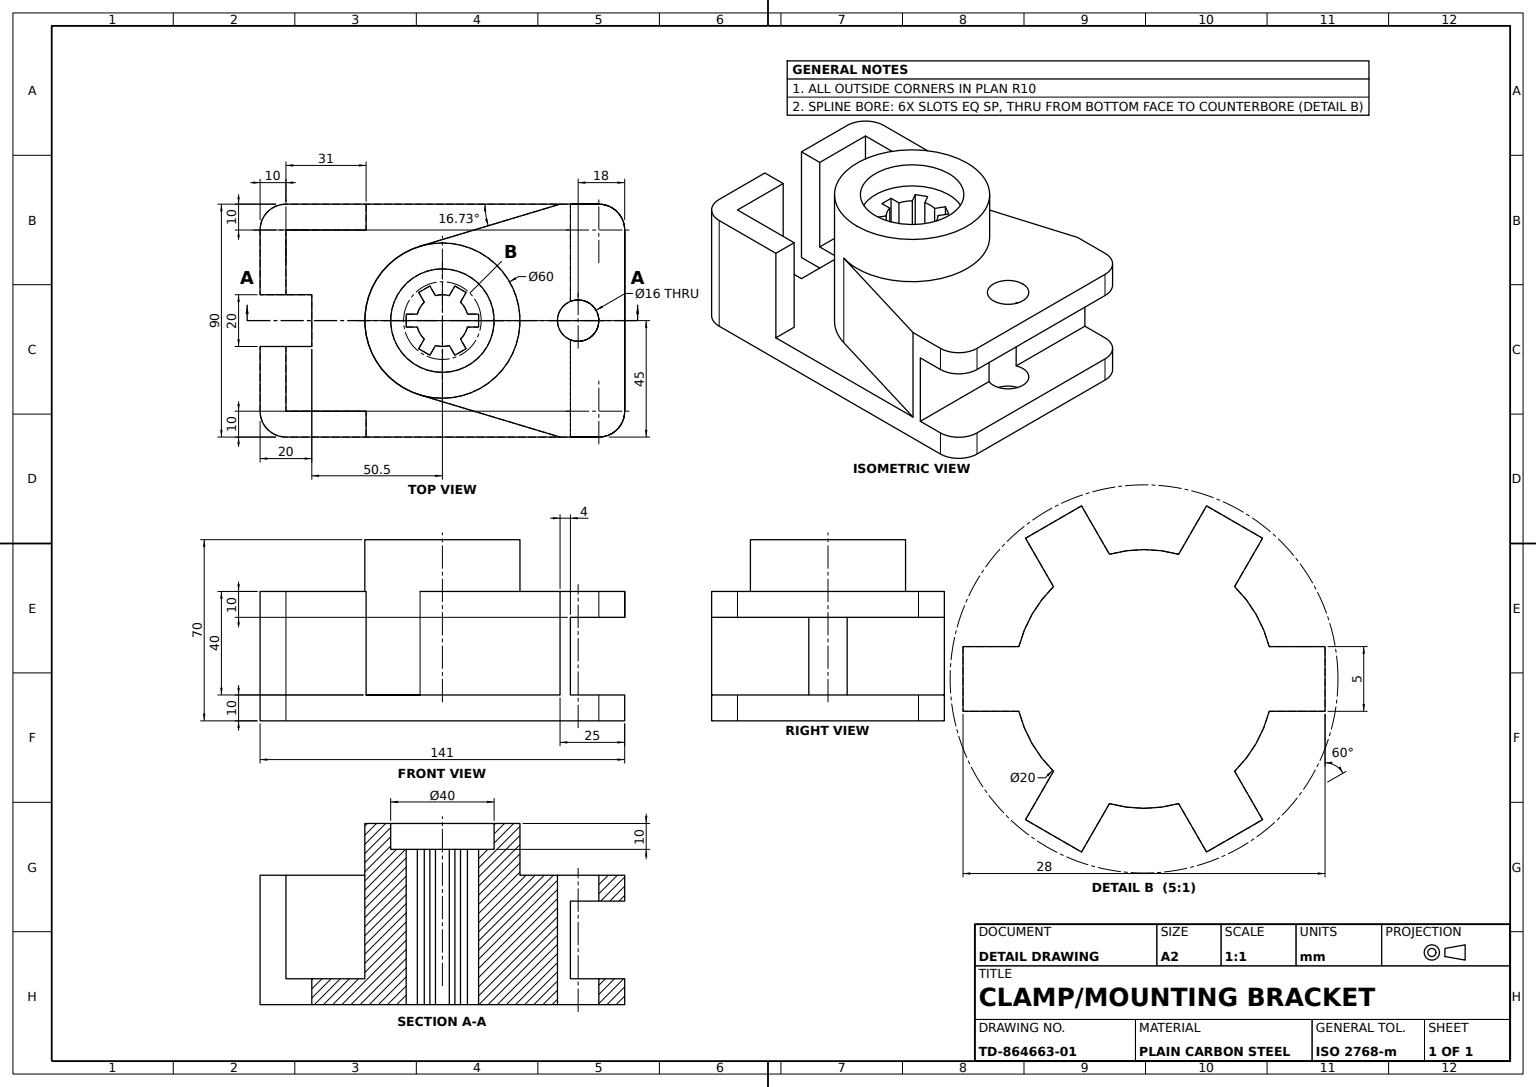
SolidWorks part; units mm, degrees
material "Plain Carbon Steel"
ref_plane "Front Plane" through (0, 0, 0) normal (0, 0, 1) x (1, 0, 0)
ref_plane "Top Plane" through (0, 0, 0) normal (0, 1, 0) x (1, 0, 0)
ref_plane "Right Plane" through (0, 0, 0) normal (1, 0, 0) x (0, 0, -1)
sketch "Base Plate Sketch" plane through (0, 0, 0) normal (0, 1, 0) x (1, 0, 0)
  line L1 (-60.5, 45) -> (60.5, 45)
  line L2 (-70.5, 35) -> (-70.5, 10)
  line L3 (-60.5, -45) -> (60.5, -45)
  line L4 (70.5, 35) -> (70.5, -35)
  line L5 (-70.5, 45) -> (70.5, -45) construction
  line L6 (-70.5, -45) -> (70.5, 45) construction
  line L7 (-70.5, -10) -> (-50.5, -10)
  line L8 (-70.5, 10) -> (-50.5, 10)
  line L9 (-70.5, -10) -> (-70.5, -35)
  line L10 (-70.5, -10) -> (-50.5, -10)
  line L12 (-50.5, -10) -> (-50.5, 10)
  arc A0 (-70.5, -35) -> (-60.5, -45) centre (-60.5, -35) ccw
  arc A1 (60.5, -45) -> (70.5, -35) centre (60.5, -35) ccw
  arc A2 (60.5, 45) -> (70.5, 35) centre (60.5, 35) cw
  arc A3 (-60.5, 45) -> (-70.5, 35) centre (-60.5, 35) ccw
  point P0 (0, 0)
  point P18 (-70.5, 0)
  point P19 (70.5, 0)
  point P23 (70.5, 10)
  dimension "D3" = 10
  dimension "D1" = 90
  dimension "D2" = 141
  dimension "D4" = 20
  dimension "D6" = 20
  dimension "D5" = 20
  dimension "D7" = 50.5
  dimension "D8" = 25
extrude "Base Plate" add sketch "Base Plate Sketch" along normal blind 10 contours L1 A3 L2 L8 L12 L7 L9 A0 L3 A1 L4 A2
sketch "Guide Wall Sketch" plane through (0, 10, 0) normal (0, 1, 0) x (1, 0, 0)
  line L0 (-60.5, 45) -> (-29.5, 45)
  line L1 (-70.5, -35) -> (-70.5, -10)
  line L2 (-60.5, 45) -> (60.5, 45) construction
  line L3 (-29.5, 45) -> (-29.5, 35)
  line L4 (-29.5, 35) -> (-60.5, 35)
  line L5 (-60.5, 35) -> (-60.5, 10)
  line L6 (-70.5, 10) -> (-50.5, 10) construction
  line L7 (-60.5, 10) -> (-70.5, 10)
  line L8 (-70.5, -10) -> (-60.5, -10)
  line L9 (-70.5, -10) -> (-50.5, -10) construction
  line L10 (-60.5, -45) -> (-29.5, -45)
  line L11 (-60.5, -45) -> (60.5, -45) construction
  line L12 (-29.5, -45) -> (-29.5, -35)
  line L13 (-29.5, -35) -> (-60.5, -35)
  line L14 (-60.5, -35) -> (-60.5, -10)
  arc A0 (-70.5, 35) -> (-60.5, 45) centre (-60.5, 35) cw
  arc A1 (-70.5, -35) -> (-60.5, -45) centre (-60.5, -35) ccw
  line M3 (60.5, 45) -> (-60.5, 45)
  arc M4 (-60.5, 45) -> (-70.5, 35) centre (-60.5, 35) ccw
  line M5 (-70.5, 35) -> (-70.5, 10)
  line M6 (-70.5, 10) -> (-50.5, 10)
  line M8 (-50.5, -10) -> (-70.5, -10)
  line M9 (-70.5, -10) -> (-70.5, -35)
  arc M10 (-70.5, -35) -> (-60.5, -45) centre (-60.5, -35) ccw
  line M11 (-60.5, -45) -> (60.5, -45)
  dimension "D1" = 31
  dimension "D2" = 31
extrude "Guide Wall" add sketch "Guide Wall Sketch" along normal blind 40 contours L5 L4 L3 M3 M4 M5 M6 | L13 L14 L12 M8 M9 M10 M11
sketch "Hub Block Sketch" plane through (0, 10, 0) normal (0, 1, 0) x (1, 0, 0)
  line L1 (45.5, -45) -> (45.5, 45)
  line L2 (70.5, 35) -> (70.5, -35) construction
  line L3 (-8.6346, 28.7305) -> (45.5, 45)
  line L4 (-8.6346, -28.7305) -> (45.5, -45)
  line L6 (-29.5, -45) -> (60.5, -45) construction
  line L7 (-29.5, 45) -> (60.5, 45) construction
  arc A0 (-8.6346, 28.7305) -> (-8.6346, -28.7305) centre (0, 0) ccw
  dimension "D1" = 60
  dimension "D2" = 25
extrude "Hub Block" add sketch "Hub Block Sketch" along normal blind 40
sketch "Clevis Ear Sketch" plane through (0, 50, 0) normal (0, 1, 0) x (1, 0, 0)
  line L0 (45.5, -45) -> (60.5, -45) construction
  line L1 (45.5, 45) -> (60.5, 45)
  line L2 (70.5, 35) -> (70.5, -35)
  line L3 (45.5, 45) -> (45.5, -45)
  line L4 (-8.6346, -28.7305) -> (45.5, -45) construction
  line L5 (-29.5, -45) -> (45.5, -45) construction
  line L6 (45.5, -45) -> (60.5, -45)
  arc A0 (60.5, 45) -> (70.5, 35) centre (60.5, 35) cw
  arc A1 (60.5, -45) -> (70.5, -35) centre (60.5, -35) ccw
  arc A2 (60.5, -45) -> (70.5, -35) centre (60.5, -35) ccw construction
  dimension "D1" = 10
extrude "Clevis Ear" add sketch "Clevis Ear Sketch" against normal blind 10
sketch "Gusset Sketch" plane through (0, 0, 45) normal (0, 0, 1) x (1, 0, 0)
  line L0 (45.5, 10) -> (60.5, 10) construction
  line L1 (45.5, 50) -> (49.5, 50)
  line L2 (45.5, 50) -> (45.5, 10)
  line L3 (45.5, 10) -> (49.5, 10)
  line L4 (49.5, 50) -> (49.5, 10)
  dimension "D1" = 4
extrude "Gusset" add sketch "Gusset Sketch" against normal blind 90
sketch "Cross Hole Sketch" plane through (0, 50, 0) normal (0, 1, 0) x (1, 0, 0)
  line L0 (70.5, -35) -> (70.5, 35) construction
  line L1 (60.5, 45) -> (45.5, 45) construction
  circle A0 centre (52.5, 0) radius 8
  dimension "D1" = 16
  dimension "D2" = 18
  dimension "D3" = 45
extrude "Cross Hole Ø16" cut sketch "Cross Hole Sketch" against normal blind 90
sketch "Hub Boss Sketch" plane through (0, 50, 0) normal (0, 1, 0) x (1, 0, 0)
  circle A0 centre (0, 0) radius 30
  dimension "D1" = 60
extrude "Hub Boss Ø60" add sketch "Hub Boss Sketch" along normal blind 20
sketch "Hub Recess Sketch" plane through (0, 70, 0) normal (0, 1, 0) x (1, 0, 0)
  circle A0 centre (0, 0) radius 20
  dimension "D1" = 40
extrude "Hub Recess Ø40" cut sketch "Hub Recess Sketch" against normal blind 10
sketch "Spline Bore Sketch" plane through (0, 60, 0) normal (0, 1, 0) x (1, 0, 0)
  line L0 (11.7367, 2.5) -> (9.6825, 2.5)
  line L1 (11.7367, -2.5) -> (14, -2.5)
  line L2 (11.7367, 2.5) -> (14, 2.5)
  line L3 (11.7367, 2.5) -> (14, 2.5)
  line L4 (14, 2.5) -> (14, -2.5)
  line L5 (14, -2.5) -> (11.7367, -2.5)
  line L6 (2.6762, -9.6353) -> (3.7033, -11.4143)
  line L7 (9.6825, -2.5) -> (11.7367, -2.5)
  line L8 (3.7033, -11.4143) -> (4.8349, -13.3744)
  line L9 (9.1651, -10.8744) -> (4.8349, -13.3744)
  line L10 (8.0334, -8.9143) -> (7.0063, -7.1353)
  line L11 (8.0334, -8.9143) -> (9.1651, -10.8744)
  line L12 (-7.0063, -7.1353) -> (-8.0334, -8.9143)
  line L13 (-8.0334, -8.9143) -> (-9.1651, -10.8744)
  line L14 (-4.8349, -13.3744) -> (-9.1651, -10.8744)
  line L15 (-3.7033, -11.4143) -> (-2.6762, -9.6353)
  line L16 (-3.7033, -11.4143) -> (-4.8349, -13.3744)
  line L17 (-9.6825, 2.5) -> (-11.7367, 2.5)
  line L18 (-11.7367, 2.5) -> (-14, 2.5)
  line L19 (-14, -2.5) -> (-14, 2.5)
  line L20 (-11.7367, -2.5) -> (-9.6825, -2.5)
  line L21 (-11.7367, -2.5) -> (-14, -2.5)
  line L22 (-2.6762, 9.6353) -> (-3.7033, 11.4143)
  line L23 (-3.7033, 11.4143) -> (-4.8349, 13.3744)
  line L24 (-9.1651, 10.8744) -> (-4.8349, 13.3744)
  line L25 (-8.0334, 8.9143) -> (-7.0063, 7.1353)
  line L26 (-8.0334, 8.9143) -> (-9.1651, 10.8744)
  line L27 (7.0063, 7.1353) -> (8.0334, 8.9143)
  line L28 (8.0334, 8.9143) -> (9.1651, 10.8744)
  line L29 (4.8349, 13.3744) -> (9.1651, 10.8744)
  line L30 (3.7033, 11.4143) -> (2.6762, 9.6353)
  line L31 (3.7033, 11.4143) -> (4.8349, 13.3744)
  arc A1 (9.6825, 2.5) -> (7.0063, 7.1353) centre (0, 0) ccw
  arc A2 (-9.6825, -2.5) -> (-7.0063, -7.1353) centre (0, 0) ccw
  arc A3 (-7.0063, 7.1353) -> (-9.6825, 2.5) centre (0, 0) ccw
  arc A4 (2.6762, 9.6353) -> (-2.6762, 9.6353) centre (0, 0) ccw
  arc A5 (7.0063, -7.1353) -> (9.6825, -2.5) centre (0, 0) ccw
  arc A6 (-2.6762, -9.6353) -> (2.6762, -9.6353) centre (0, 0) ccw
  point P3 (0, -2.5)
  point P4 (76.2883, 0)
  point P5 (76.2883, -2.5)
  point P6 (0, 2.5)
  point P7 (76.2883, 2.5)
  dimension "D1" = 6
  dimension "D6" = 20
  dimension "D2" = 5
  dimension "D4" = 2.2633
  dimension "D3" = 2.2633
  dimension "D5" = 11.7367
  dimension "D7" = 2.5
extrude "Spline Bore 6x" cut sketch "Spline Bore Sketch" against normal blind 90 contours L15 A6 L6 L8 L9 L11 L10 A5 L7 L1 L4 L2 L0 A1 L27 L28 L29 L31 L30 A4 L22 L23 L24 L26 L25 A3 L17 L18 L19 L21 L20 A2 L12 L13 L14 L16
